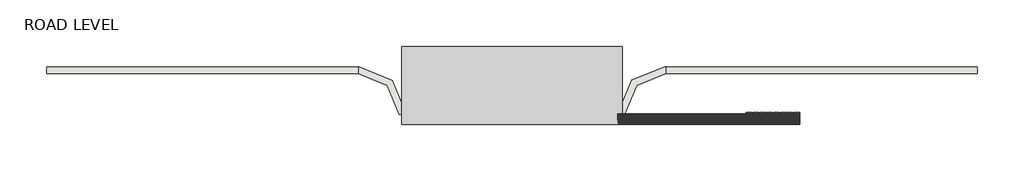
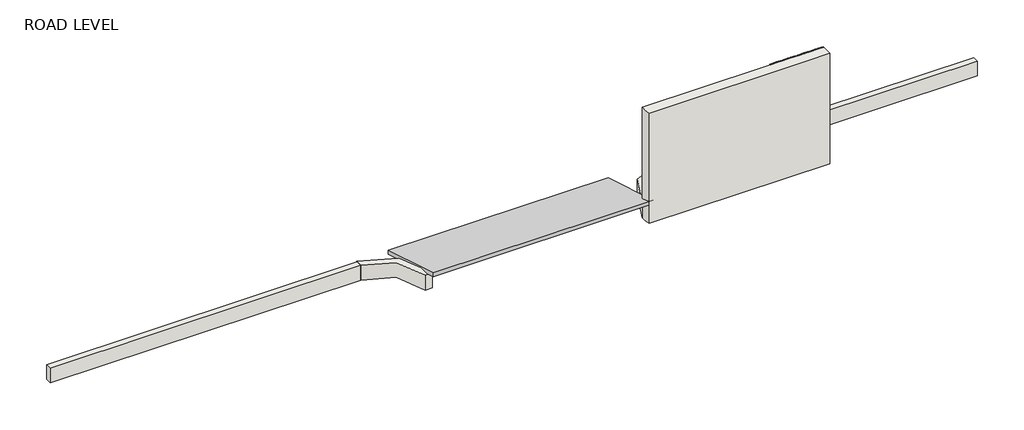
# One storey: 5 walls, 1 proxy, 1 ramp.
"""IFC4 building model written with IfcOpenShell, lengths in millimetres."""

from ifc_helpers import new_model, si_unit, frame, origin, origin_with_axes, place, context, project, spatial, polyline, circle_curve, outline, extrude, transform, mapped, element, save
from ifc_brep_helpers import plane_surface, cylinder_surface, revolved_surface, advanced_brep
from components import generic_models_1_generic_models_1_37e6f81f, ramp_3_deb929ff

model = new_model("IFC4")

# Units and contexts
model_context = context("Model", 3, world=origin())
ifc_project = project(units=[si_unit("LENGTHUNIT", "METRE", prefix="MILLI")], contexts=[model_context])

# Site, building, storey
site = spatial("IfcSite", under=ifc_project)
building = spatial("IfcBuilding", under=site)
storey = spatial("IfcBuildingStorey", under=building, Name="ROAD LEVEL", Elevation=0.0)

# Proxy
placement = place(None, origin())
generic_models_1_generic_models_1_shape = generic_models_1_generic_models_1_37e6f81f(model_context)
element("IfcBuildingElementProxy", 1, Name="Generic Models 1 : Generic Models 1", ObjectType="Generic Models 1 : Generic Models 1", at=placement, inside=storey, context=model_context, shape_type="MappedRepresentation", body=[
    mapped(generic_models_1_generic_models_1_shape, transform((0.0, 0.0, 0.0), x_axis=(1.0, 0.0, 0.0), y_axis=(0.0, 1.0, 0.0), z_axis=(0.0, 0.0, 1.0))),
])

# Ramp
ramp_3_shape = ramp_3_deb929ff(model_context)
element("IfcRamp", 2, ObjectType="Ramp 3", at=placement, inside=storey, context=model_context, shape_type="MappedRepresentation", body=[
    mapped(ramp_3_shape, transform((0.0, 0.0, 0.0), x_axis=(1.0, 0.0, 0.0), y_axis=(0.0, 1.0, 0.0), z_axis=(0.0, 0.0, 1.0))),
])

# Walls
element("IfcWall", 3, ObjectType="Generic - 8\"", at=placement, inside=storey, context=model_context, shape_type="AdvancedBrep", body=[
    advanced_brep(
    [(-15452.5378983, -5561.5027976, 0.0), (-11913.168705, -5561.5027976, 0.0), (-11913.168705, -5561.5027976, 914.4), (-11913.168705, -5561.5027976, 2286.0), (-12116.368705, -5561.5027976, 2286.0), (-15452.5378983, -5561.5027976, 2286.0), (-15472.2781146, -5358.3027976, 0.0), (-15472.2781146, -5358.3027976, 304.8), (-15472.2781146, -5358.3027976, 2286.0), (-11913.168705, -5358.3027976, 2286.0), (-11913.168705, -5358.3027976, 0.0), (-15332.5666839, -5358.3027976, 0.0)],
    [
        (0, 1),
        (1, 2),
        (2, 3),
        (3, 4),
        (4, 5),
        (5, 0),
        (6, 7),
        (7, 8),
        (8, 9),
        (9, 10),
        (10, 11),
        (11, 6),
        (0, 6, circle_curve(frame((-14530.956205, -5369.4152976, 0.0), z_axis=(0.0, 0.0, -1.0), x_axis=(-1.0, 0.0, 0.0)), 941.3875)),
        (10, 1),
        (3, 9),
        (8, 5, circle_curve(frame((-14530.956205, -5369.4152976, 2286.0), z_axis=(0.0, 0.0, 1.0), x_axis=(-1.0, 0.0, 0.0)), 941.3875)),
    ],
    [
        plane_surface(frame((-15380.268705, -5561.5027976, 0.0), z_axis=(0.0, -1.0, 0.0), x_axis=(1.0, 0.0, 0.0))),
        plane_surface(frame((-15380.268705, -5358.3027976, 0.0), z_axis=(0.0, 1.0, 0.0), x_axis=(-1.0, 0.0, 0.0))),
        plane_surface(frame((-15397.7835386, -5561.5027976, 0.0), z_axis=(0.0, 0.0, -1.0), x_axis=(0.0, 1.0, 0.0))),
        plane_surface(frame((-12014.768705, -5561.5027976, 2286.0), z_axis=(0.0, 0.0, 1.0), x_axis=(0.0, 1.0, 0.0))),
        plane_surface(frame((-11913.168705, -5568.6238659, 914.4), z_axis=(1.0, 0.0, 0.0), x_axis=(0.0, 1.0, 0.0))),
        cylinder_surface(frame((-14530.956205, -5369.4152976, 0.0), z_axis=(0.0, 0.0, 1.0), x_axis=(-1.0, 0.0, 0.0)), 941.3875),
    ],
    [
        (0, [[1, 2, 3, 4, 5, 6]]),
        (1, [[7, 8, 9, 10, 11, 12]]),
        (2, [[-1, 13, -12, -11, 14]]),
        (3, [[-5, -4, 15, -9, 16]]),
        (4, [[-3, -2, -14, -10, -15]]),
        (5, [[-6, -16, -8, -7, -13]]),
    ],
),
])
element("IfcWall", 4, ObjectType="Interior - 4 7/8\" Partition (1-hr) 2", at=placement, inside=storey, context=model_context, shape_type="SweptSolid", body=[
    extrude(outline(polyline([(-26619.768705, -4443.9027976), (-20534.881205, -4443.9027976), (-20534.881205, -4567.7277976), (-26619.768705, -4567.7277976), (-26619.768705, -4443.9027976)])), origin_with_axes(), (0.0, 0.0, 1.0), 304.8),
])
element("IfcWall", 5, ObjectType="Interior - 4 7/8\" Partition (1-hr) 2", at=placement, inside=storey, context=model_context, shape_type="SweptSolid", body=[
    extrude(outline(polyline([(-8446.068705, -4567.7277976), (-14530.956205, -4567.7277976), (-14530.956205, -4443.9027976), (-8446.068705, -4443.9027976), (-8446.068705, -4567.7277976)])), origin_with_axes(), (0.0, 0.0, 1.0), 304.8),
])
element("IfcWall", 6, ObjectType="Interior - 5 1/2\" Partition (1-hr)", at=placement, inside=storey, context=model_context, shape_type="AdvancedBrep", body=[
    advanced_brep(
    [(-19593.493705, -5369.4152976, 304.8), (-20534.881205, -4428.0277976, 304.8), (-20534.881205, -4443.9027976, 304.8), (-20534.881205, -4567.7277976, 304.8), (-19733.193705, -5369.4152976, 304.8), (-19593.493705, -5369.4152976, 0.0), (-19733.193705, -5369.4152976, 0.0), (-20534.881205, -4567.7277976, 0.0), (-20534.881205, -4443.9027976, 0.0), (-20534.881205, -4428.0277976, 0.0)],
    [
        (0, 1, circle_curve(frame((-20534.881205, -5369.4152976, 304.8), z_axis=(0.0, 0.0, 1.0), x_axis=(1.0, 0.0, 0.0)), 941.3875)),
        (1, 2),
        (2, 3),
        (3, 4, circle_curve(frame((-20534.881205, -5369.4152976, 304.8), z_axis=(0.0, 0.0, -1.0), x_axis=(1.0, 0.0, 0.0)), 801.6875)),
        (4, 0),
        (5, 6),
        (6, 7, circle_curve(frame((-20534.881205, -5369.4152976, 0.0), z_axis=(0.0, 0.0, 1.0), x_axis=(1.0, 0.0, 0.0)), 801.6875)),
        (7, 8),
        (8, 9),
        (9, 5, circle_curve(frame((-20534.881205, -5369.4152976, 0.0), z_axis=(0.0, 0.0, -1.0), x_axis=(1.0, 0.0, 0.0)), 941.3875)),
        (0, 5),
        (9, 1),
        (7, 3),
        (6, 4),
    ],
    [
        plane_surface(frame((-19593.493705, -5369.4152976, 304.8), z_axis=(0.0, 0.0, 1.0), x_axis=(0.0, 1.0, 0.0))),
        plane_surface(frame((-19593.493705, -5369.4152976, 0.0), z_axis=(0.0, 0.0, -1.0), x_axis=(0.0, -1.0, 0.0))),
        cylinder_surface(frame((-20534.881205, -5369.4152976, 0.0), z_axis=(0.0, 0.0, 1.0), x_axis=(1.0, 0.0, 0.0)), 941.3875),
        plane_surface(frame((-20534.881205, -4428.0277976, 304.8), z_axis=(-1.0, 0.0, 0.0), x_axis=(0.0, 0.0, -1.0))),
        revolved_surface(polyline([(-19733.193705, -5369.4152976, 0.0), (-19733.193705, -5369.4152976, 304.8)]), (-20534.881205, -5369.4152976, 0.0), (0.0, 0.0, -1.0)),
        plane_surface(frame((-19733.193705, -5369.4152976, 304.8), z_axis=(0.0, -1.0, 0.0), x_axis=(0.0, 0.0, -1.0))),
    ],
    [
        (0, [[1, 2, 3, 4, 5]]),
        (1, [[6, 7, 8, 9, 10]]),
        (2, [[-1, 11, -10, 12]]),
        (3, [[-3, -2, -12, -9, -8, 13]]),
        (4, [[-4, -13, -7, 14]]),
        (5, [[-5, -14, -6, -11]]),
    ],
),
])
element("IfcWall", 7, ObjectType="Interior - 5 1/2\" Partition (1-hr)", at=placement, inside=storey, context=model_context, shape_type="AdvancedBrep", body=[
    advanced_brep(
    [(-15332.5666839, -5358.3027976, 304.8), (-14530.956205, -4567.7277976, 304.8), (-14530.956205, -4443.9027976, 304.8), (-14530.956205, -4428.0277976, 304.8), (-15472.2781146, -5358.3027976, 304.8), (-15332.5666839, -5358.3027976, 0.0), (-15472.2781146, -5358.3027976, 0.0), (-14530.956205, -4428.0277976, 0.0), (-14530.956205, -4443.9027976, 0.0), (-14530.956205, -4567.7277976, 0.0)],
    [
        (0, 1, circle_curve(frame((-14530.956205, -5369.4152976, 304.8), z_axis=(0.0, 0.0, -1.0), x_axis=(-1.0, 0.0, 0.0)), 801.6875)),
        (1, 2),
        (2, 3),
        (3, 4, circle_curve(frame((-14530.956205, -5369.4152976, 304.8), z_axis=(0.0, 0.0, 1.0), x_axis=(-1.0, 0.0, 0.0)), 941.3875)),
        (4, 0),
        (5, 6),
        (6, 7, circle_curve(frame((-14530.956205, -5369.4152976, 0.0), z_axis=(0.0, 0.0, -1.0), x_axis=(-1.0, 0.0, 0.0)), 941.3875)),
        (7, 8),
        (8, 9),
        (9, 5, circle_curve(frame((-14530.956205, -5369.4152976, 0.0), z_axis=(0.0, 0.0, 1.0), x_axis=(-1.0, 0.0, 0.0)), 801.6875)),
        (0, 5),
        (9, 1),
        (7, 3),
        (6, 4),
    ],
    [
        plane_surface(frame((-15332.643705, -5369.4152976, 304.8), z_axis=(0.0, 0.0, 1.0), x_axis=(0.0, 1.0, 0.0))),
        plane_surface(frame((-15332.643705, -5369.4152976, 0.0), z_axis=(0.0, 0.0, -1.0), x_axis=(0.0, -1.0, 0.0))),
        revolved_surface(polyline([(-15332.643705, -5369.4152976, 0.0), (-15332.643705, -5369.4152976, 304.8)]), (-14530.956205, -5369.4152976, 0.0), (0.0, 0.0, -1.0)),
        plane_surface(frame((-14530.956205, -4567.7277976, 304.8), z_axis=(1.0, 0.0, 0.0), x_axis=(0.0, 0.0, -1.0))),
        cylinder_surface(frame((-14530.956205, -5369.4152976, 0.0), z_axis=(0.0, 0.0, 1.0), x_axis=(-1.0, 0.0, 0.0)), 941.3875),
        plane_surface(frame((-15380.268705, -5358.3027976, 0.0), z_axis=(0.0, -1.0, 0.0), x_axis=(-1.0, 0.0, 0.0))),
    ],
    [
        (0, [[1, 2, 3, 4, 5]]),
        (1, [[6, 7, 8, 9, 10]]),
        (2, [[-1, 11, -10, 12]]),
        (3, [[-3, -2, -12, -9, -8, 13]]),
        (4, [[-4, -13, -7, 14]]),
        (5, [[-5, -14, -6, -11]]),
    ],
),
])

save(model, "model.ifc")

# Revit data of these elements
# Type "Ramp 3"
#   Assembly Code = "B1010600"
#   built-in parameter 1008304 = 0.25 (stored number, unit not read)
#   built-in parameter 1008303 = 30 (stored number, unit not read)
#   built-in parameter 1008301 = 3.333 (stored number, unit not read)
#   Function = 0
#   built-in parameter 1008308 = Vinyl Composition Tile
# Type "Generic - 8\""
#   Assembly Code = "B2010"
#   Layers, outside or top first: 0' - 8" no material (function 1)
# Type "Interior - 4 7/8\" Partition (1-hr) 2"
#   Assembly Code = "C1010145"
# Type "Interior - 5 1/2\" Partition (1-hr)"
#   Assembly Code = "C1010145"
#   Layers, outside or top first: 0' - 0 5/8" "Gypsum Wall Board" (function 5); 0' - 3 5/8" "Metal Stud Layer" (function 1); 0' - 0 5/8" "Gypsum Wall Board" (function 5); 0' - 0 5/8" "Gypsum Wall Board" (function 5)
# Element 1 (IfcBuildingElementProxy, "Generic Models 1 : Generic Models 1")
#   Phase Created = New Construction
#   Materials on its faces: "Wood Planks"
# Element 2 (IfcRamp, "Ramp 3")
#   built-in parameter 1007275 = "DN"
#   built-in parameter 1007272 = "UP"
#   Width = 3' - 0"
#   built-in parameter 1007276 = 1
#   built-in parameter 1007274 = 1
#   built-in parameter 1007273 = 1
#   built-in parameter 1007271 = 1
#   Phase Created = New Construction
#   Materials on its faces: "Vinyl Composition Tile"
# Element 3 (IfcWall, "Generic - 8\"")
#   Top Offset = 0' - 0"
#   Base Offset = 0' - 0"
#   Unconnected Height = 7' - 6"
#   wall height = 7' - 6"
#   Phase Created = New Construction
#   Base Constraint = ROAD LEVEL
#   Materials on its faces: "Default Wall", "Gypsum Wall Board"
# Elements 4, 5 (IfcWall, "Interior - 4 7/8\" Partition (1-hr) 2")
#   Top Offset = 0' - 0"
#   Base Offset = 0' - 0"
#   Unconnected Height = 1' - 0"
#   wall height = 1' - 0"
#   Phase Created = New Construction
#   Base Constraint = ROAD LEVEL
#   Materials on its faces: "Default Wall", "Gypsum Wall Board"
# Elements 6, 7 (IfcWall, "Interior - 5 1/2\" Partition (1-hr)")
#   Top Offset = 0' - 0"
#   Base Offset = 0' - 0"
#   Unconnected Height = 1' - 0"
#   wall height = 1' - 0"
#   Phase Created = New Construction
#   Materials on its faces: "Default Wall", "Gypsum Wall Board"
# Materials
#   "Vinyl Composition Tile": class "Generic", colour RGB 179 160 124, transparency 0, Description = "Vinyl Composition Tile", Cost = 0
#   "Gypsum Wall Board": class "Generic", colour RGB 228 228 228, transparency 0, Description = "Gypsum Wall Board", Cost = 0
#   "Metal Stud Layer": class "Metal", colour RGB 199 199 199, transparency 0, Description = "Light gauge steel framing, thermal air layer", Cost = 0
#   "Wood Planks": class "Wood", colour RGB 129 72 39, transparency 0, Description = "Physical material.", Cost = 0
#   "Default Wall": colour RGB 128 128 128, transparency 0, Cost = 0
